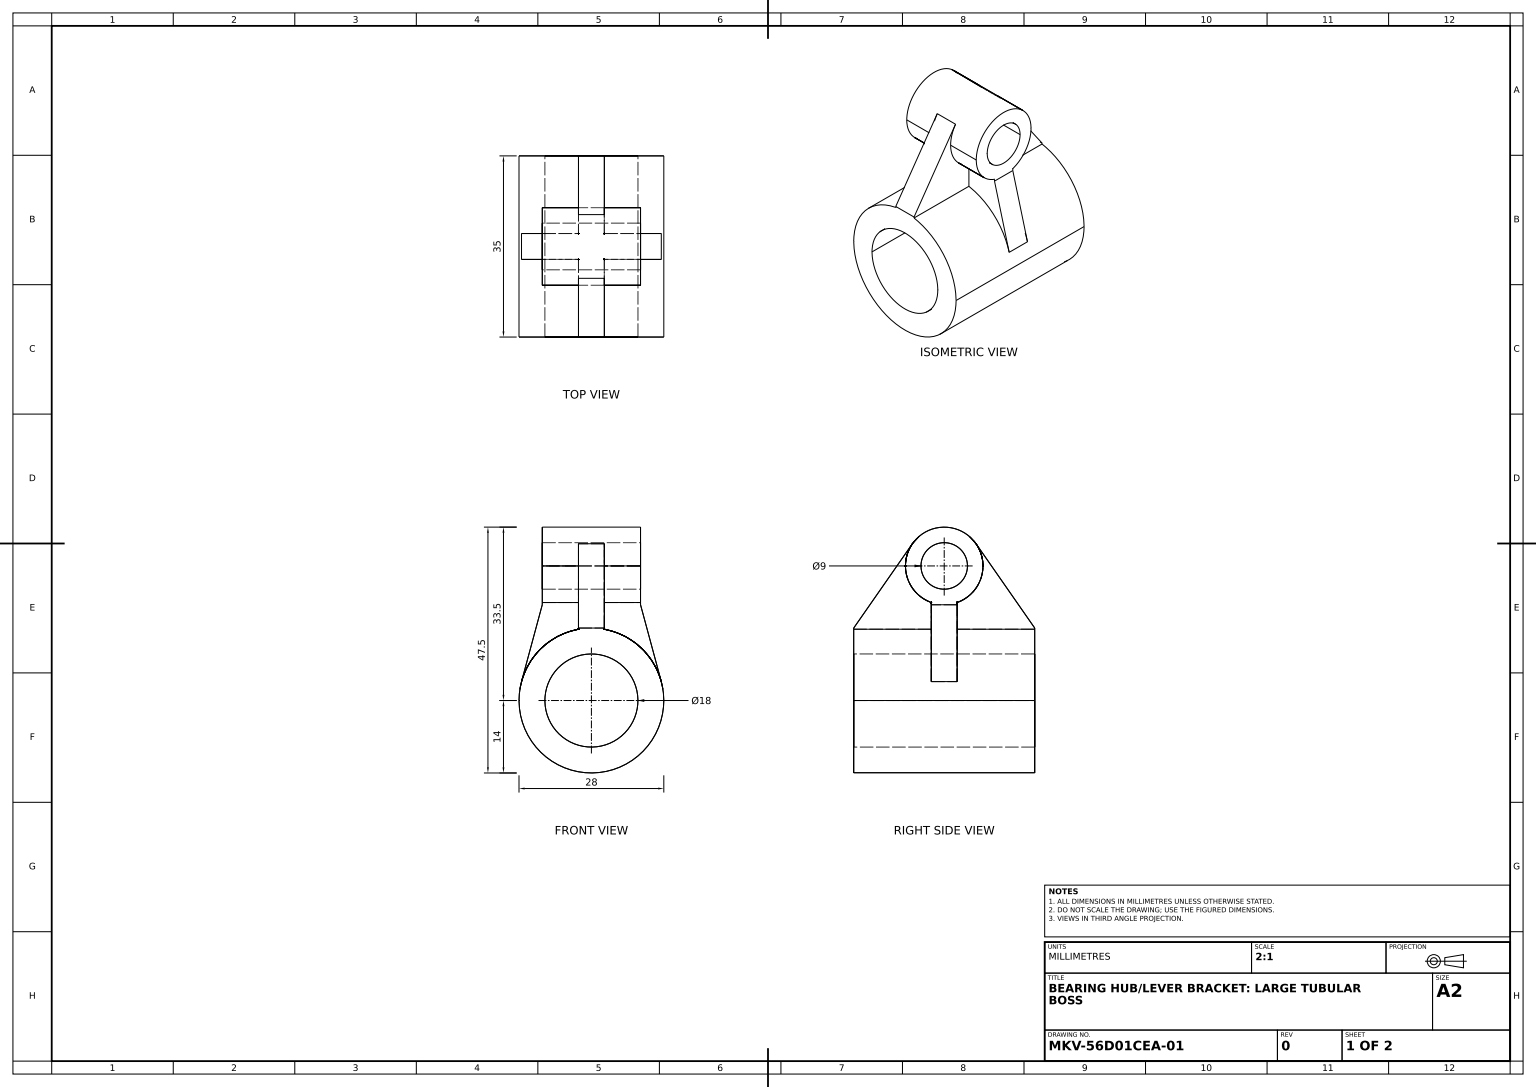
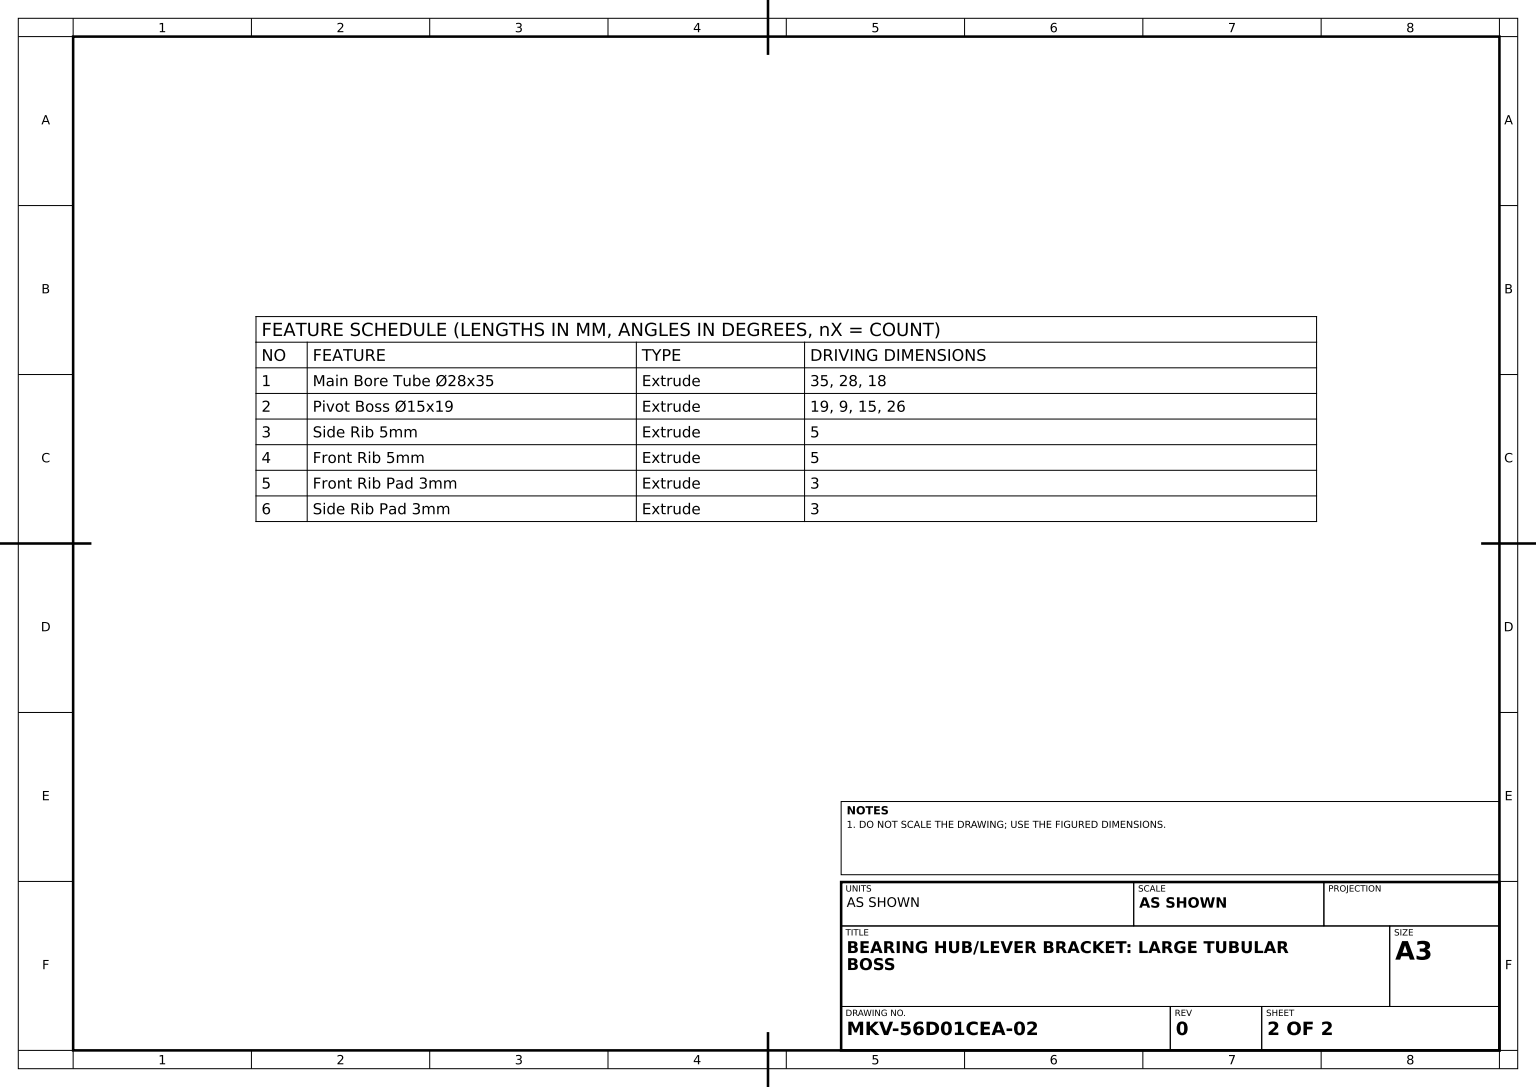
SolidWorks part; units mm, degrees
material "Plain Carbon Steel"
ref_plane "Front Plane" through (0, 0, 0) normal (0, 0, 1) x (1, 0, 0)
ref_plane "Top Plane" through (0, 0, 0) normal (0, 1, 0) x (1, 0, 0)
ref_plane "Right Plane" through (0, 0, 0) normal (1, 0, 0) x (0, 0, -1)
sketch "Main Bore Profile Ø28-Ø18" plane through (0, 0, 0) normal (0, 0, 1) x (1, 0, 0)
  circle A2 centre (0, 0) radius 14
  circle A3 centre (0, 0) radius 9
  dimension "D1" = 28
  dimension "D2" = 18
extrude "Main Bore Tube Ø28x35" add sketch "Main Bore Profile Ø28-Ø18" along normal mid plane 35
sketch "Pivot Boss Profile Ø15-Ø9" plane through (0, 0, 0) normal (1, 0, 0) x (0, 0, -1)
  line L0 (0, 0) -> (0, 26) construction
  circle A0 centre (0, 26) radius 7.5
  circle A1 centre (0, 26) radius 4.5
  dimension "D1" = 9
  dimension "D2" = 15
  dimension "D3" = 26
extrude "Pivot Boss Ø15x19" add sketch "Pivot Boss Profile Ø15-Ø9" along normal mid plane 19 separate body
sketch "Side Rib Profile" plane through (0, 0, 0) normal (1, 0, 0) x (0, 0, -1)
  line L0 (-17.5, 14) -> (-6.154, 30.287)
  line L1 (17.5, 14) -> (6.154, 30.287)
  line L2 (-17.5, 14) -> (17.5, 14)
  circle A0 centre (0, 26) radius 7.5 construction
  arc A1 (-6.154, 30.287) -> (6.154, 30.287) centre (0, 26) ccw
extrude "Side Rib 5mm" add sketch "Side Rib Profile" along normal mid plane 5
sketch "Front Rib Profile" plane through (0, 0, 0) normal (0, 0, 1) x (1, 0, 0)
  line L0 (-13.5146, 3.6547) -> (-9.5, 18.5)
  line L1 (-9.5, 18.5) -> (9.5, 18.5)
  line L2 (9.5, 18.5) -> (13.5146, 3.6547)
  circle A0 centre (0, 0) radius 14 construction
  arc A1 (13.5146, 3.6547) -> (-13.5146, 3.6547) centre (0, 0) ccw
extrude "Front Rib 5mm" add sketch "Front Rib Profile" along normal mid plane 5 separate body
sketch "Front Rib Pad Profile" plane through (0, 18.5, 0) normal (0, 1, 0) x (1, 0, 0)
  line L1 (-9.5, 2.5) -> (9.5, 2.5)
  line L2 (-9.5, 2.5) -> (-9.5, -2.5)
  line L3 (-9.5, -2.5) -> (9.5, -2.5)
  line L4 (9.5, 2.5) -> (9.5, -2.5)
extrude "Front Rib Pad 3mm" add sketch "Front Rib Pad Profile" along normal blind 3
sketch "Side Rib Pad Profile" plane through (0, 14, 0) normal (0, -1, 0) x (1, 0, 0)
  line L1 (-2.5, 17.5) -> (2.5, 17.5)
  line L2 (-2.5, 17.5) -> (-2.5, -17.5)
  line L3 (-2.5, -17.5) -> (2.5, -17.5)
  line L4 (2.5, 17.5) -> (2.5, -17.5)
extrude "Side Rib Pad 3mm" add sketch "Side Rib Pad Profile" along normal blind 3
